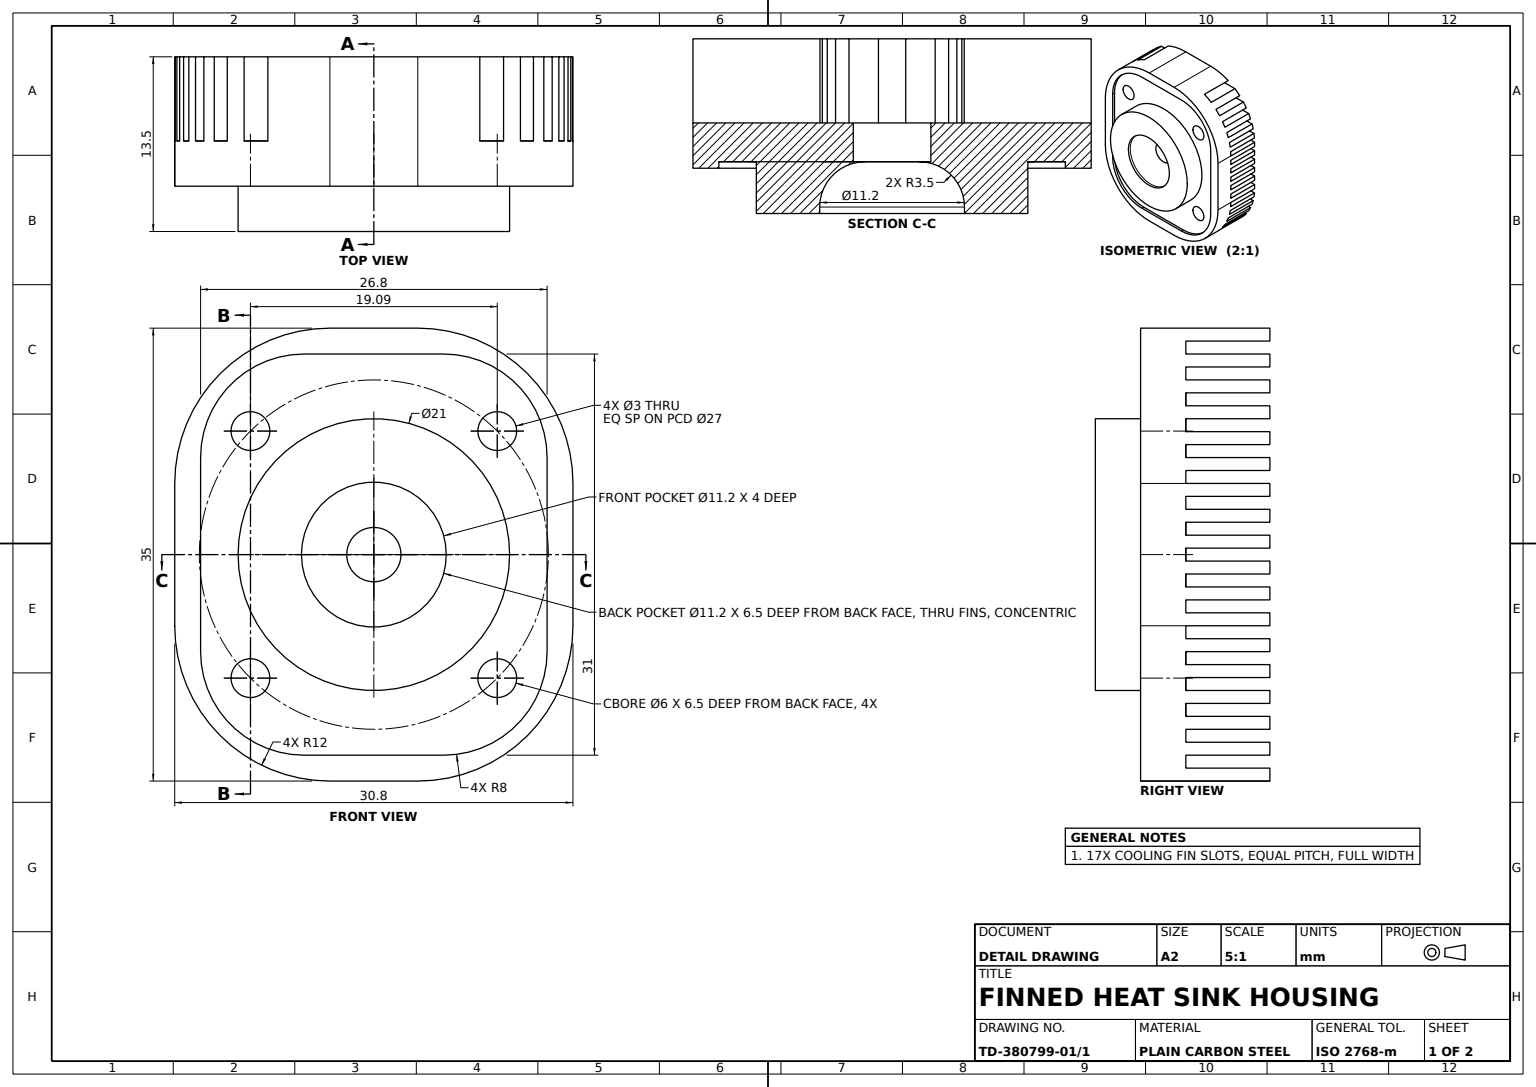
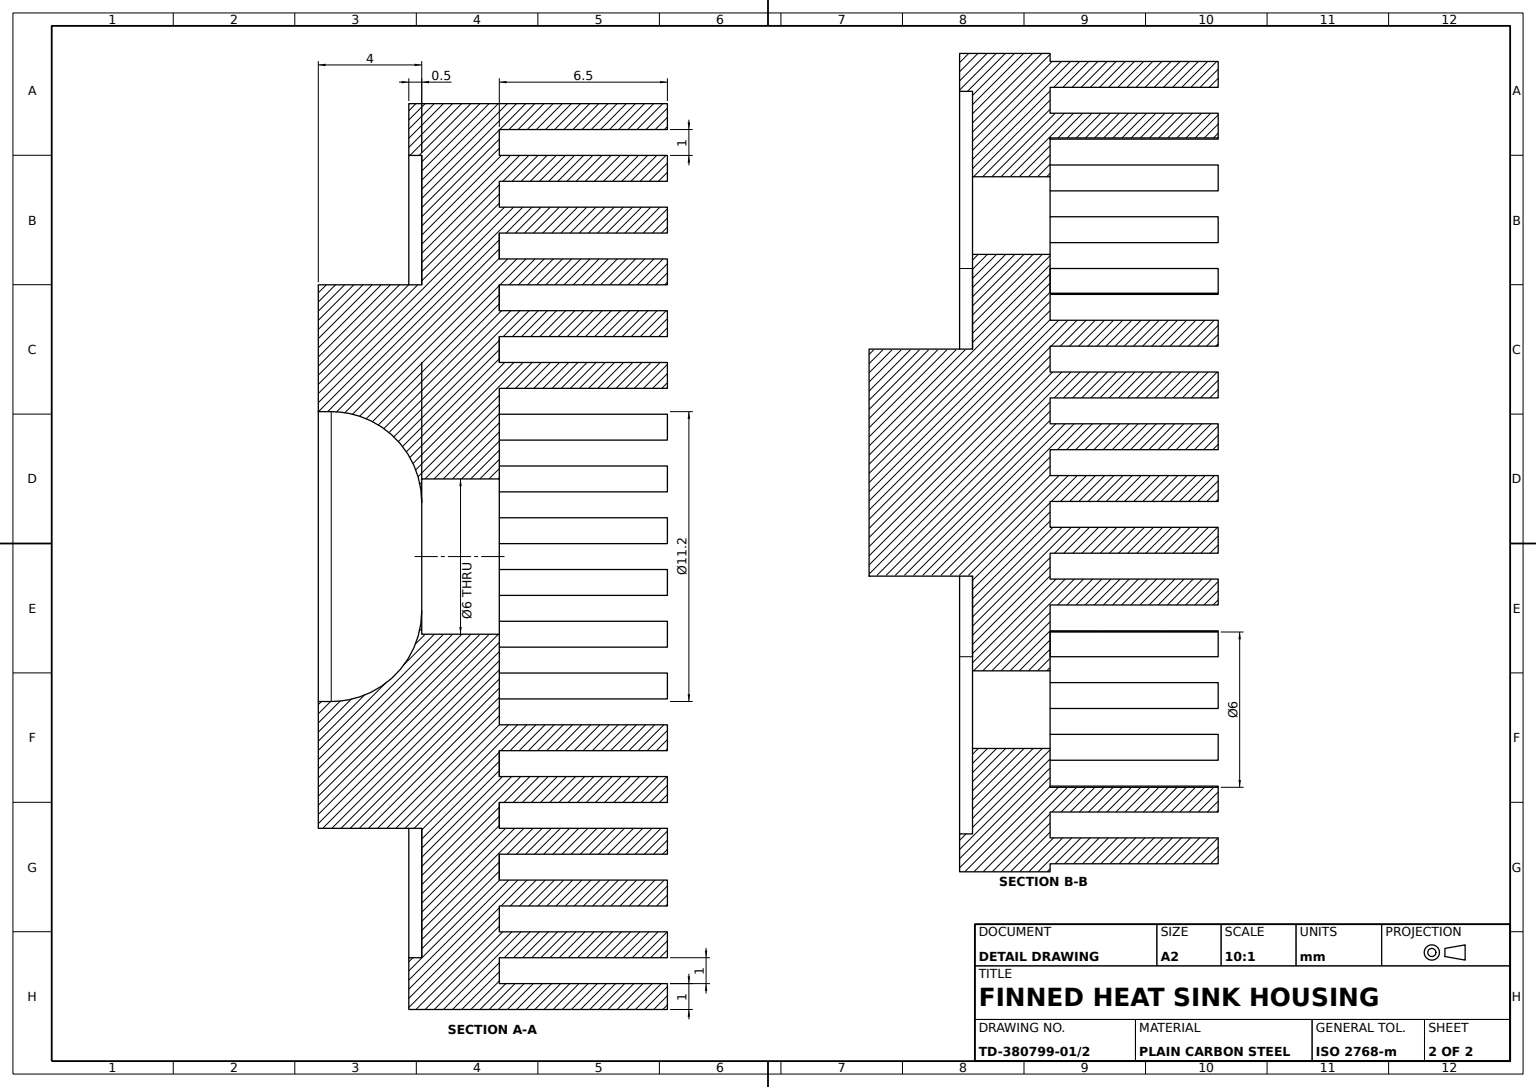
from build123d import *

# Parameters (mm, degrees)
HEAD_BASE_BODY_DEPTH       = 10
FACE_RECESS_0_5MM_DEPTH    = 0.5
HUB_SKETCH_R               = 10.5
HUB_SKETCH_R_2             = 5.6
RAISED_HUB_21_DEPTH        = 4
RECESS_FILLET_R3_5_R       = 3.5
CENTRE_BORE_SKETCH_R       = 3
CENTRE_BORE_6_DEPTH        = 3.5
COOLING_FIN_SLOTS_SKETCH_W = 6.5
COOLING_FIN_SLOTS_SKETCH_H = 1
COOLING_FIN_SLOTS_DEPTH    = 27.93807714
MOUNTING_HOLES_SKETCH_R    = 1.5
MOUNTING_HOLES_3_DEPTH     = 3.5
HUB_BORE_SKETCH_R          = 5.6
HUB_BORE_11_2_DEPTH        = 25.339474111
SIDE_CUT_SKETCH_R          = 3
SIDE_CUT_6X6_DEPTH         = 25.339474111


with BuildPart() as part:
    # Head Outline Sketch → Head Base Body (new body)
    with BuildSketch(Plane.XY):
        with BuildLine():
            Line((-3.4, -17.5), (3.4, -17.5))
            ThreePointArc((3.4, -17.5), (11.885281374, -13.985281374), (15.4, -5.5))
            Line((15.4, -5.5), (15.4, 5.5))
            ThreePointArc((15.4, 5.5), (11.885281374, 13.985281374), (3.4, 17.5))
            Line((3.4, 17.5), (-3.4, 17.5))
            ThreePointArc((-3.4, 17.5), (-11.885281374, 13.985281374), (-15.4, 5.5))
            Line((-15.4, 5.5), (-15.4, -5.5))
            ThreePointArc((-15.4, -5.5), (-11.885281374, -13.985281374), (-3.4, -17.5))
        make_face()
    extrude(amount=HEAD_BASE_BODY_DEPTH)

    # Face Recess Sketch → Face Recess 0.5mm (cut)
    with BuildSketch(Plane.XY.offset(10)):
        with BuildLine():
            Line((-13.4, 7.5), (-13.4, -7.5))
            ThreePointArc((-13.4, -7.5), (-11.056854249, -13.156854249), (-5.4, -15.5))
            Line((-5.4, -15.5), (5.4, -15.5))
            ThreePointArc((5.4, -15.5), (11.056854249, -13.156854249), (13.4, -7.5))
            Line((13.4, -7.5), (13.4, 7.5))
            ThreePointArc((13.4, 7.5), (11.056854249, 13.156854249), (5.4, 15.5))
            Line((5.4, 15.5), (-5.4, 15.5))
            ThreePointArc((-5.4, 15.5), (-11.056854249, 13.156854249), (-13.4, 7.5))
        make_face()
    extrude(amount=-FACE_RECESS_0_5MM_DEPTH, mode=Mode.SUBTRACT)

    # Hub Sketch → Raised Hub Ø21 (add)
    with BuildSketch(Plane.XY.offset(9.5)):
        Circle(HUB_SKETCH_R)
        Circle(HUB_SKETCH_R_2, mode=Mode.SUBTRACT)
    extrude(amount=RAISED_HUB_21_DEPTH)

    # Recess Fillet R3.5
    recess_fillet_r3_5_edges = [part.edges().sort_by_distance(p)[0] for p in [
        (-5.6, 0, 9.5),
    ]]
    fillet(recess_fillet_r3_5_edges, radius=RECESS_FILLET_R3_5_R)

    # Centre Bore Sketch → Centre Bore Ø6 (cut)
    with BuildSketch(Plane.XY.offset(9.5)):
        Circle(CENTRE_BORE_SKETCH_R)
    extrude(amount=-CENTRE_BORE_6_DEPTH, mode=Mode.SUBTRACT)

    # Cooling Fin Slots Sketch → Cooling Fin Slots (cut, symmetric)
    with BuildSketch(Plane(origin=(0, 0, 0), x_dir=(0, 0, -1), z_dir=(1, 0, 0))):
        with Locations((-3.25, 2)):
            Rectangle(COOLING_FIN_SLOTS_SKETCH_W, COOLING_FIN_SLOTS_SKETCH_H)
        with Locations((-3.25, 0)):
            Rectangle(COOLING_FIN_SLOTS_SKETCH_W, COOLING_FIN_SLOTS_SKETCH_H)
        with Locations((-3.25, 4)):
            Rectangle(COOLING_FIN_SLOTS_SKETCH_W, COOLING_FIN_SLOTS_SKETCH_H)
        with Locations((-3.25, 6)):
            Rectangle(COOLING_FIN_SLOTS_SKETCH_W, COOLING_FIN_SLOTS_SKETCH_H)
        with Locations((-3.25, 8)):
            Rectangle(COOLING_FIN_SLOTS_SKETCH_W, COOLING_FIN_SLOTS_SKETCH_H)
        with Locations((-3.25, 10)):
            Rectangle(COOLING_FIN_SLOTS_SKETCH_W, COOLING_FIN_SLOTS_SKETCH_H)
        with Locations((-3.25, 12)):
            Rectangle(COOLING_FIN_SLOTS_SKETCH_W, COOLING_FIN_SLOTS_SKETCH_H)
        with Locations((-3.25, 14)):
            Rectangle(COOLING_FIN_SLOTS_SKETCH_W, COOLING_FIN_SLOTS_SKETCH_H)
        with Locations((-3.25, 16)):
            Rectangle(COOLING_FIN_SLOTS_SKETCH_W, COOLING_FIN_SLOTS_SKETCH_H)
    cooling_fin_slots = extrude(amount=COOLING_FIN_SLOTS_DEPTH, both=True, mode=Mode.SUBTRACT)

    # Cooling Fin Slots Mirror: Cooling Fin Slots across plane
    add(cooling_fin_slots.mirror(Plane.ZX), mode=Mode.SUBTRACT)

    # Mounting Holes Sketch → Mounting Holes Ø3 (cut)
    with BuildSketch(Plane.XY.offset(9.5)):
        with Locations((-9.545, 9.545)):
            Circle(MOUNTING_HOLES_SKETCH_R)
        with Locations((9.545, 9.545)):
            Circle(MOUNTING_HOLES_SKETCH_R)
        with Locations(Location((9.545, -9.545, 0), (0, 0, 1.719131321))):
            Circle(MOUNTING_HOLES_SKETCH_R)
        with Locations(Location((-9.545, -9.545, 0), (0, 0, 1.719131321))):
            Circle(MOUNTING_HOLES_SKETCH_R)
    extrude(amount=-MOUNTING_HOLES_3_DEPTH, mode=Mode.SUBTRACT)

    # Hub Bore Sketch → Hub Bore Ø11.2 (cut, through all)
    with BuildSketch(Plane(origin=(0, 0, 6.5), x_dir=(-1, 0, 0), z_dir=(0, 0, -1))):
        with Locations(Location((0, 0, 0), (0, 0, 180))):
            Circle(HUB_BORE_SKETCH_R)
    extrude(amount=HUB_BORE_11_2_DEPTH, mode=Mode.SUBTRACT)

    # Side Cut Sketch → Side Cut 6x6 (cut, through all)
    with BuildSketch(Plane(origin=(0, 0, 6.5), x_dir=(-1, 0, 0), z_dir=(0, 0, -1))):
        with Locations((-9.545, 9.545)):
            Circle(SIDE_CUT_SKETCH_R)
        with Locations((9.545, 9.545)):
            Circle(SIDE_CUT_SKETCH_R)
        with Locations((-9.545, -9.545)):
            Circle(SIDE_CUT_SKETCH_R)
        with Locations((9.545, -9.545)):
            Circle(SIDE_CUT_SKETCH_R)
    extrude(amount=SIDE_CUT_6X6_DEPTH, mode=Mode.SUBTRACT)


solid = part.part
